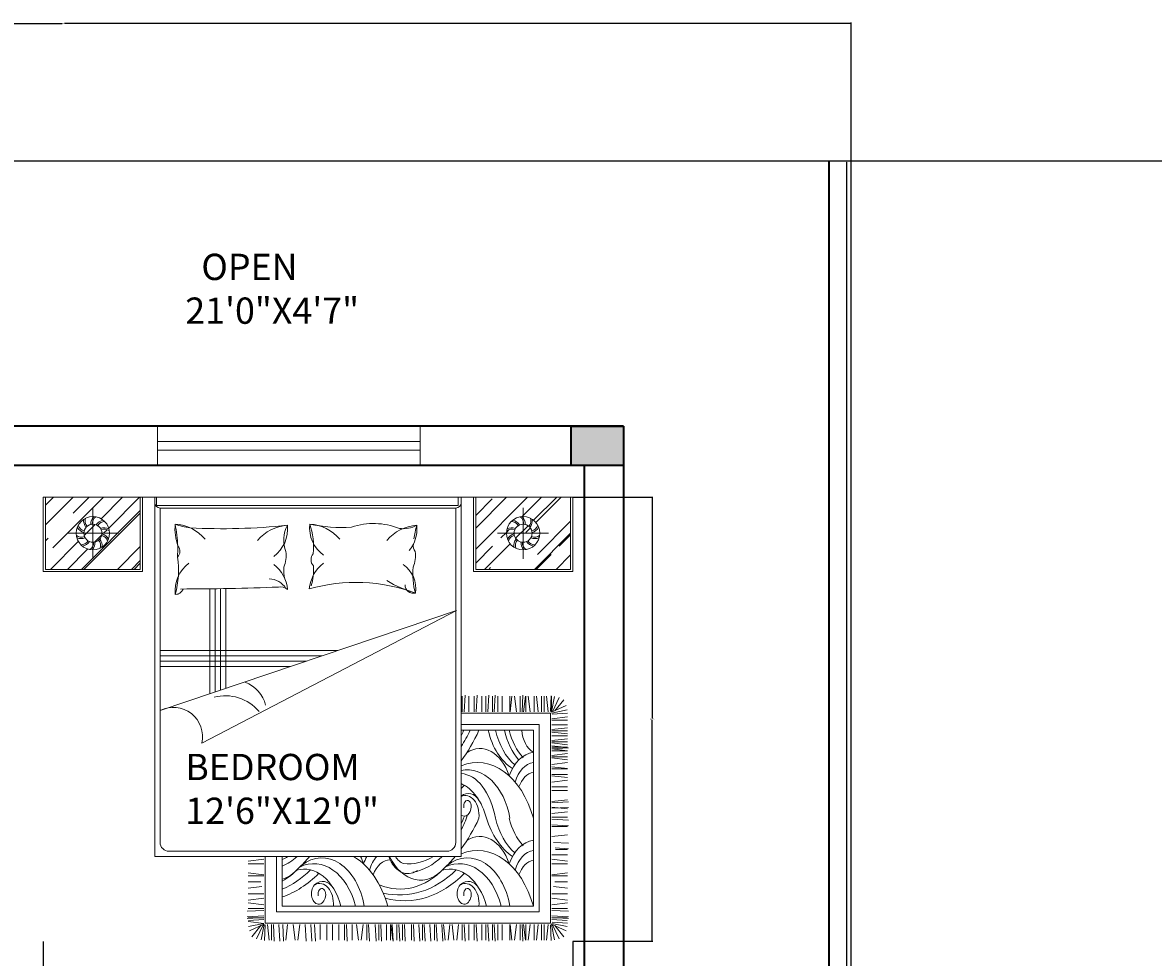
# Model space of a CAD drawing. Units: inches. Extents: x 1602 to 2642, y 1463 to 2270.
# Tile 4 of 5: x 1854 to 2113, y 1919 to 2132. Entities that reach past the tile are written whole.
import ezdxf

# ---------------------------------------------------------------- set-up
doc = ezdxf.new("R2010")
doc.units = ezdxf.units.IN
for name, color, linetype, lineweight in [('A-ANNO-DIMS', 2, 'Continuous', 18), ('A-AREA-IDEN', 7, 'Continuous', 18), ('A-COLS', 7, 'Continuous', 35), ('A-FURN', 8, 'Continuous', 13), ('A-GLAZ', 4, 'Continuous', 18), ('A-WALL', 7, 'Continuous', 35), ('C-PROP', 7, 'Continuous', 25)]:
    doc.layers.add(name, color=color, linetype=linetype, lineweight=lineweight)
doc.styles.get("Standard").update_dxf_attribs({"font": 'arial.ttf'})
doc.dimstyles.get("Standard").update_dxf_attribs({"dimtxt": 0.18, "dimasz": 0.18, "dimexe": 0.18, "dimexo": 0.0625, "dimgap": 0.09, "dimtad": 0, "dimtih": 1, "dimtoh": 1, "dimdec": 4, "dimzin": 0, "dimdsep": 46, "dimtxsty": 'Standard', "dimcen": 0.09, "dimadec": 0, "dimazin": 0, "dimtfac": 1, "dimtdec": 4, "dimtofl": 0, "dimtmove": 0, "dimatfit": 3, "dimfxl": 1, "dimtolj": 1, "dimtzin": 0, "dimarcsym": 0})

# ---------------------------------------------------------------- blocks, each defined once
blk = doc.blocks.new('A$C64B41DC1')
for p, q in [((0, 2.5079), (2.9903, 2.5079)), ((0, 2.0879), (0, 2.5079)), ((0.012, 2.4618), (0.0581, 2.5079)), ((0.012, 2.3515), (0.1684, 2.5079)), ((0.012, 2.0999), (0.012, 2.5079)), ((0.0543, 2.2213), (0.3409, 2.5079)), ((0.1689, 2.4179), (0.2589, 2.5079)), ((0.3265, 2.386), (0.4484, 2.5079)), ((0.3699, 2.3332), (0.5445, 2.5079)), ((0.548, 2.5079), (0.548, 2.0999)), ((0.56, 2.5079), (0.56, 2.0879)), ((0.6301, 2.5079), (0.6301, 0.4779)), ((0.6401, 2.461), (0.6401, 2.5079)), ((0.6401, 2.5079), (2.344, 2.5079)), ((2.344, 2.5079), (2.3601, 2.5079)), ((2.344, 2.5079), (2.344, 2.461)), ((2.3601, 2.5079), (2.3601, 2.4761)), ((2.3601, 0.4779), (2.3601, 2.5079)), ((2.4303, 2.5079), (2.4303, 2.0879)), ((2.4423, 2.5079), (2.4423, 2.0999)), ((2.4423, 2.3333), (2.6169, 2.5079)), ((2.4423, 2.2145), (2.7357, 2.5079)), ((2.4423, 2.404), (2.5354, 2.4971)), ((2.705, 2.398), (2.8149, 2.5079)), ((2.7691, 2.3772), (2.8998, 2.5079)), ((2.7819, 2.3646), (2.9252, 2.5079)), ((2.9783, 2.0999), (2.9783, 2.5079)), ((2.9903, 2.0879), (2.9903, 2.5079)), ((0.2157, 2.0999), (0.548, 2.4322)), ((0.2804, 2.1597), (0.2804, 2.4481)), ((2.344, 2.461), (0.6401, 2.461)), ((0.6601, 2.4461), (1.4951, 2.4461)), ((0.6601, 2.4461), (0.6601, 0.5579)), ((1.4951, 2.4461), (0.6697, 2.4461)), ((2.3301, 2.4461), (1.4951, 2.4461)), ((2.3301, 0.5579), (2.3301, 2.4461)), ((2.7099, 2.1597), (2.7099, 2.4481)), ((0.2299, 2.0999), (0.548, 2.418)), ((2.7914, 2.1846), (2.9783, 2.3715)), ((0.1362, 2.3039), (0.4246, 2.3039)), ((0.2311, 2.2906), (0.2937, 2.3532)), ((0.3405, 2.3039), (0.3605, 2.3238)), ((2.8541, 2.3039), (2.5657, 2.3039)), ((2.5849, 2.2779), (2.6158, 2.3088)), ((2.6158, 2.3088), (2.6313, 2.3243)), ((2.6674, 2.2756), (2.7382, 2.3464)), ((2.7249, 2.3076), (2.7512, 2.3339)), ((2.7746, 2.0999), (2.9783, 2.3036)), ((0.012, 2.261), (0.0275, 2.2765)), ((0.0404, 2.0999), (0.1982, 2.2578)), ((0.2905, 2.2539), (0.3304, 2.2938)), ((2.4918, 2.0999), (2.6366, 2.2447)), ((2.9144, 2.2312), (2.9783, 2.2951)), ((0.1365, 2.0999), (0.251, 2.2144)), ((0.4194, 2.0999), (0.548, 2.2285)), ((2.4423, 2.1353), (2.5382, 2.2312)), ((2.7831, 2.0999), (2.8678, 2.1846)), ((2.8962, 2.0999), (2.9783, 2.182)), ((0.4986, 2.0999), (0.548, 2.1493)), ((0.5127, 2.0999), (0.548, 2.1352)), ((2.5172, 2.0999), (2.5269, 2.1096)), ((0.56, 2.0879), (0, 2.0879)), ((0.548, 2.0999), (0.012, 2.0999)), ((2.4303, 2.0879), (2.9903, 2.0879)), ((2.4423, 2.0999), (2.9783, 2.0999)), ((0.9415, 1.9902), (0.9415, 1.3975)), ((0.9715, 1.9906), (0.9715, 1.4076)), ((1.0015, 1.991), (1.0015, 1.4177)), ((1.0315, 1.9916), (1.0315, 1.4279)), ((2.3349, 1.8678), (0.6613, 1.3029)), ((0.8956, 1.1191), (2.3349, 1.8678)), ((1.6636, 1.6412), (0.6601, 1.6412)), ((1.5748, 1.6112), (0.6601, 1.6112)), ((2.3665, 1.295), (2.3665, 1.3839)), ((2.377, 1.295), (2.3822, 1.3891)), ((2.4032, 1.295), (2.4032, 1.3839)), ((2.4346, 1.295), (2.4346, 1.3839)), ((2.4451, 1.295), (2.4503, 1.3891)), ((2.4774, 1.2957), (2.4774, 1.3837)), ((2.5, 1.295), (2.5, 1.3839)), ((2.5105, 1.295), (2.5157, 1.3891)), ((2.5367, 1.295), (2.5367, 1.3839)), ((2.5471, 1.295), (2.5524, 1.3891)), ((2.5681, 1.295), (2.5681, 1.3839)), ((2.5918, 1.295), (2.5918, 1.3839)), ((2.6346, 1.2957), (2.6346, 1.3837)), ((2.6362, 1.2957), (2.6467, 1.3839)), ((2.6729, 1.295), (2.6624, 1.3839)), ((2.6938, 1.295), (2.6938, 1.3839)), ((2.7043, 1.295), (2.7095, 1.3891)), ((2.7127, 1.2957), (2.7232, 1.3839)), ((2.7253, 1.295), (2.7253, 1.3839)), ((2.7494, 1.295), (2.7389, 1.3839)), ((2.7718, 1.295), (2.7718, 1.3839)), ((2.7959, 1.295), (2.7854, 1.3839)), ((2.8146, 1.2957), (2.8146, 1.3837)), ((2.8146, 1.2957), (2.8146, 1.3837)), ((2.8282, 1.295), (2.8282, 1.3839)), ((2.8282, 1.295), (2.8282, 1.3839)), ((2.8523, 1.295), (2.8418, 1.3839)), ((2.8523, 1.295), (2.8418, 1.3839)), ((2.8653, 1.2966), (2.8688, 1.3861)), ((2.8711, 1.2957), (2.8711, 1.3837)), ((2.8711, 1.2957), (2.8875, 1.3822)), ((2.8765, 1.2958), (2.9132, 1.3758)), ((2.8893, 1.3011), (2.9394, 1.3636)), ((2.3601, 1.2873), (2.8639, 1.2873)), ((2.8639, 1.2873), (2.8639, 0.1018)), ((2.8713, 1.2927), (2.954, 1.3315)), ((2.8717, 1.2884), (2.9588, 1.3058)), ((2.8744, 1.2817), (2.9603, 1.2869)), ((2.3601, 1.2233), (2.7999, 1.2233)), ((2.7999, 1.2233), (2.7999, 0.1658)), ((2.8716, 1.2565), (2.9605, 1.2669)), ((2.8716, 1.2212), (2.9605, 1.2212)), ((2.8723, 1.2489), (2.9603, 1.2489)), ((2.3601, 1.1913), (2.7679, 1.1912)), ((2.7679, 1.1912), (2.7679, 0.1978)), ((2.8716, 1.1947), (2.9605, 1.2052)), ((2.8716, 1.181), (2.9605, 1.1705)), ((2.8716, 1.1595), (2.9605, 1.1595)), ((2.8723, 1.1872), (2.9603, 1.1872)), ((2.8716, 1.133), (2.9605, 1.1435)), ((2.8716, 1.1193), (2.9605, 1.1088)), ((2.8716, 1.1035), (2.9605, 1.093)), ((2.8716, 1.0965), (2.9605, 1.0965)), ((2.8716, 1.086), (2.9657, 1.0913)), ((2.8723, 1.1255), (2.9603, 1.1255)), ((2.8723, 1.0858), (2.9605, 1.0753)), ((2.8716, 1.0756), (2.9605, 1.0756)), ((2.8716, 1.0491), (2.9605, 1.0596)), ((2.8716, 1.0354), (2.9605, 1.0249)), ((2.8723, 1.0416), (2.9603, 1.0416)), ((2.8723, 0.9987), (2.9605, 1.0092)), ((2.8723, 0.985), (2.9605, 0.9745)), ((2.8723, 0.9735), (2.9603, 0.9735)), ((2.8716, 0.9346), (2.9605, 0.9241)), ((2.8723, 0.9408), (2.9603, 0.9408)), ((2.8723, 0.8979), (2.9605, 0.9084)), ((2.8723, 0.8726), (2.9603, 0.8726)), ((2.8723, 0.8505), (2.9603, 0.8505)), ((2.8716, 0.7885), (2.9605, 0.799)), ((2.8716, 0.7818), (2.9657, 0.787)), ((2.8716, 0.7503), (2.9657, 0.7556)), ((2.8716, 0.7204), (2.9605, 0.7309)), ((2.8723, 0.7571), (2.9605, 0.7466)), ((2.8716, 0.6995), (2.9605, 0.6995)), ((2.8716, 0.689), (2.9657, 0.6838)), ((2.8716, 0.6576), (2.9657, 0.6523)), ((2.8716, 0.6471), (2.9605, 0.6471)), ((2.8716, 0.5903), (2.9605, 0.6007)), ((2.882, 0.5582), (2.9657, 0.5536)), ((2.8909, 0.5263), (2.9657, 0.5222)), ((2.8928, 0.5169), (2.9605, 0.5169)), ((0.6301, 0.4779), (2.3601, 0.4779)), ((0.7101, 0.5079), (2.2801, 0.5079)), ((1.2465, 0.4625), (1.1576, 0.452)), ((1.2542, 0.1018), (1.2542, 0.4779)), ((1.3182, 0.1658), (1.3182, 0.4779)), ((1.3502, 0.1978), (1.3502, 0.4779)), ((2.8716, 0.4877), (2.9603, 0.4877)), ((2.8716, 0.4625), (2.9605, 0.452)), ((1.2465, 0.3746), (1.1576, 0.3851)), ((1.2465, 0.4365), (1.1577, 0.4365)), ((2.8716, 0.4365), (2.9603, 0.4365)), ((2.8716, 0.3746), (2.9605, 0.3851)), ((1.2465, 0.3684), (1.1577, 0.3684)), ((1.2285, 0.3357), (1.1577, 0.3357)), ((2.8716, 0.3684), (2.9603, 0.3684)), ((2.8896, 0.3357), (2.9603, 0.3357)), ((1.2355, 0.3092), (1.1576, 0.3)), ((1.2457, 0.2676), (1.1577, 0.2676)), ((2.8723, 0.2676), (2.9603, 0.2676)), ((2.8826, 0.3092), (2.9605, 0.3)), ((1.2457, 0.2423), (1.1576, 0.2319)), ((1.2465, 0.2057), (1.1576, 0.2161)), ((2.7679, 0.1978), (1.3502, 0.1978)), ((2.8716, 0.2057), (2.9605, 0.2161)), ((2.8723, 0.2423), (2.9605, 0.2319)), ((1.2465, 0.1742), (1.1524, 0.169)), ((1.2465, 0.1428), (1.1524, 0.1376)), ((1.2465, 0.1334), (1.1524, 0.1281)), ((1.2465, 0.1847), (1.1576, 0.1847)), ((1.2465, 0.1323), (1.1576, 0.1323)), ((1.2465, 0.1323), (1.1576, 0.1323)), ((2.7999, 0.1658), (1.3182, 0.1658)), ((2.8716, 0.1847), (2.9605, 0.1847)), ((2.8716, 0.1742), (2.9657, 0.169)), ((2.8716, 0.1428), (2.9657, 0.1376)), ((2.8716, 0.1334), (2.9657, 0.1281)), ((2.8716, 0.1323), (2.9605, 0.1323)), ((1.2465, 0.1), (1.1576, 0.1105)), ((1.2465, 0.1229), (1.1588, 0.1168)), ((1.2464, 0.1007), (1.1592, 0.0833)), ((1.2468, 0.0964), (1.1641, 0.0576)), ((1.2288, 0.088), (1.1787, 0.0255)), ((1.2415, 0.0933), (1.2049, 0.0133)), ((1.247, 0.0934), (1.2306, 0.0069)), ((1.2527, 0.0925), (1.2493, 0.003)), ((2.8639, 0.1018), (1.2542, 0.1018)), ((1.2658, 0.0941), (1.2762, 0.0052)), ((1.2899, 0.0941), (1.2899, 0.0052)), ((1.2999, 0.0941), (1.3051, 0)), ((1.3313, 0.0941), (1.3365, 0)), ((1.3523, 0.0941), (1.3575, 0)), ((1.3804, 0.0941), (1.3699, 0.0052)), ((1.4119, 0.0934), (1.4223, 0.0052)), ((1.4485, 0.0941), (1.438, 0.0052)), ((1.48, 0.0941), (1.4852, 0)), ((1.5114, 0.0941), (1.5166, 0)), ((1.5323, 0.0941), (1.5376, 0)), ((1.5638, 0.0941), (1.5638, 0.0105)), ((1.6021, 0.0941), (1.6021, 0.0052)), ((1.6336, 0.0941), (1.6336, 0.0052)), ((1.6702, 0.0941), (1.6702, 0.0052)), ((1.7017, 0.0941), (1.7017, 0.0052)), ((1.7122, 0.0941), (1.7174, 0)), ((1.7445, 0.0934), (1.7445, 0.0054)), ((1.7698, 0.0934), (1.7803, 0.0052)), ((1.8065, 0.0941), (1.796, 0.0052)), ((1.8274, 0.0941), (1.8274, 0.0052)), ((1.8379, 0.0941), (1.8431, 0)), ((1.8746, 0.0941), (1.8798, 0)), ((1.8955, 0.0941), (1.8955, 0.0052)), ((1.906, 0.0941), (1.9113, 0)), ((1.9384, 0.0934), (1.9384, 0.0054)), ((1.9609, 0.0941), (1.9609, 0.0052)), ((1.9636, 0.0934), (1.9741, 0.0052)), ((1.9714, 0.0941), (1.9766, 0)), ((1.9976, 0.0941), (1.9976, 0.0052)), ((2.0081, 0.0941), (2.0133, 0)), ((2.029, 0.0941), (2.029, 0.0052)), ((2.0395, 0.0941), (2.0447, 0)), ((2.0797, 0.0941), (2.0797, 0.0052)), ((2.0902, 0.0941), (2.0954, 0)), ((2.1216, 0.0941), (2.1269, 0)), ((2.1412, 0.0941), (2.1412, 0.0052)), ((2.1517, 0.0941), (2.1569, 0)), ((2.1831, 0.0941), (2.1884, 0)), ((2.2093, 0.0941), (2.2093, 0.0052)), ((2.2198, 0.0941), (2.225, 0)), ((2.2512, 0.0941), (2.2565, 0)), ((2.2603, 0.0934), (2.2707, 0.0052)), ((2.2969, 0.0941), (2.2864, 0.0052)), ((2.3089, 0.0934), (2.3193, 0.0052)), ((2.3455, 0.0941), (2.3351, 0.0052)), ((2.3665, 0.0941), (2.3665, 0.0052)), ((2.377, 0.0941), (2.3822, 0)), ((2.4032, 0.0941), (2.4032, 0.0052)), ((2.4346, 0.0941), (2.4346, 0.0052)), ((2.4451, 0.0941), (2.4503, 0)), ((2.4774, 0.0934), (2.4774, 0.0054)), ((2.5, 0.0941), (2.5, 0.0052)), ((2.5105, 0.0941), (2.5157, 0)), ((2.5367, 0.0941), (2.5367, 0.0052)), ((2.5471, 0.0941), (2.5524, 0)), ((2.5681, 0.0941), (2.5681, 0.0052)), ((2.5918, 0.0941), (2.5918, 0.0052)), ((2.6346, 0.0934), (2.6346, 0.0054)), ((2.6362, 0.0934), (2.6467, 0.0052)), ((2.6729, 0.0941), (2.6624, 0.0052)), ((2.6938, 0.0941), (2.6938, 0.0052)), ((2.7043, 0.0941), (2.7095, 0)), ((2.7127, 0.0934), (2.7232, 0.0052)), ((2.7253, 0.0941), (2.7253, 0.0052)), ((2.7494, 0.0941), (2.7389, 0.0052)), ((2.7718, 0.0941), (2.7718, 0.0052)), ((2.7959, 0.0941), (2.7854, 0.0052)), ((2.8146, 0.0934), (2.8146, 0.0054)), ((2.8282, 0.0941), (2.8282, 0.0052)), ((2.8523, 0.0941), (2.8418, 0.0052)), ((2.8653, 0.0925), (2.8688, 0.003)), ((2.8711, 0.0934), (2.8875, 0.0069)), ((2.8713, 0.0964), (2.954, 0.0576)), ((2.8716, 0.1229), (2.9593, 0.1168)), ((2.8717, 0.1007), (2.9588, 0.0833)), ((2.8744, 0.1074), (2.9603, 0.1022)), ((2.8765, 0.0933), (2.9132, 0.0133)), ((2.8893, 0.088), (2.9394, 0.0255))]:
    blk.add_line(p, q)
at = {"ltscale": 10}
for p, q in [((1.4859, 1.5812), (0.6601, 1.5812)), ((1.397, 1.5512), (0.6601, 1.5512))]:
    blk.add_line(p, q, dxfattribs=at)
for centre, radius in [((0.2804, 2.3039), 0.0942), ((2.7099, 2.3039), 0.0942), ((0.2804, 2.3039), 0.051), ((2.7099, 2.3039), 0.051)]:
    blk.add_circle(centre, radius)
for centre, radius, start, end in [((0.6601, 2.4761), 0.03, 180, 270), ((2.3301, 2.4761), 0.03, 270, 0), ((0.2887, 2.3745), 0.0605, 172.17003, 218.48975), ((0.2828, 2.3731), 0.0462, 160.30017, 220.53802), ((0.3286, 2.3561), 0.0605, 136.17003, 182.48975), ((0.3231, 2.3585), 0.0462, 124.30017, 184.53802), ((0.3501, 2.3178), 0.0605, 100.17003, 146.48975), ((0.347, 2.323), 0.0462, 88.30017, 148.53802), ((2.6433, 2.323), 0.0462, 31.46198, 91.69983), ((2.6402, 2.3178), 0.0605, 33.51025, 79.82997), ((2.6672, 2.3585), 0.0462, 355.46198, 55.69983), ((2.6617, 2.3561), 0.0605, 357.51025, 43.82997), ((2.7075, 2.3731), 0.0462, 319.46198, 19.69983), ((2.7016, 2.3745), 0.0605, 321.51025, 7.82997), ((0.2457, 2.3659), 0.0605, 208.17003, 254.48975), ((0.2417, 2.3614), 0.0462, 196.30017, 256.53802), ((0.3449, 2.2742), 0.0605, 64.17003, 110.48975), ((0.3455, 2.2802), 0.0462, 52.30017, 112.53802), ((0.3151, 2.2419), 0.0605, 28.17003, 74.48975), ((1.0526, 2.3302), 0.3085, 175.30484, 198.69419), ((-0.8702, 2.0941), 1.6364, 4.80985, 9.18918), ((0.8579, 2.6278), 0.2948, 247.51785, 264.26696), ((0.728, 2.111), 0.245, 40.4189, 85.9871), ((1.0164, 5.7096), 3.3803, 266.81337, 276.16021), ((1.3963, 2.1044), 0.245, 94.0129, 139.5811), ((1.1858, 2.3288), 0.1943, 306.5711, 5.88998), ((1.5348, 2.2652), 0.1767, 151.77364, 201.69827), ((1.6986, 2.3355), 0.1943, 174.11002, 233.4289), ((1.1481, 2.2311), 0.3783, 353.49469, 19.18669), ((1.6871, 3.192), 0.8561, 257.74383, 273.62843), ((1.4882, 2.111), 0.245, 40.4189, 85.9871), ((1.8674, 1.9709), 0.3878, 68.20259, 108.9817), ((2.1269, 2.1044), 0.245, 94.0129, 139.5811), ((2.0342, 2.4856), 0.1563, 261.59582, 298.90918), ((1.9165, 2.3288), 0.1943, 333.73715, 5.88998), ((2.6058, 2.2028), 0.517, 163.60457, 172.3273), ((2.6448, 2.2802), 0.0462, 67.46198, 127.69983), ((2.6454, 2.2742), 0.0605, 69.51025, 115.82997), ((2.6752, 2.2419), 0.0605, 105.51025, 151.82997), ((2.7486, 2.3614), 0.0462, 283.46198, 343.69983), ((2.7446, 2.3659), 0.0605, 285.51025, 331.82997), ((0.2153, 2.3276), 0.0462, 232.30017, 292.53802), ((0.2158, 2.3336), 0.0605, 244.17003, 290.48975), ((0.2138, 2.2848), 0.0462, 268.30017, 328.53802), ((0.2107, 2.29), 0.0605, 280.17003, 326.48975), ((0.2377, 2.2493), 0.0462, 304.30017, 4.53802), ((0.2322, 2.2517), 0.0605, 316.17003, 2.48975), ((0.2779, 2.2347), 0.0462, 340.30017, 40.53802), ((0.272, 2.2333), 0.0605, 352.17003, 38.48975), ((0.3191, 2.2464), 0.0462, 16.30017, 76.53802), ((1.9165, 2.3288), 0.1943, 320.94042, 333.73715), ((2.1347, 2.2313), 0.0459, 165.35061, 223.26844), ((2.6712, 2.2464), 0.0462, 103.46198, 163.69983), ((2.7182, 2.2333), 0.0605, 141.51025, 187.82997), ((2.7123, 2.2347), 0.0462, 139.46198, 199.69983), ((2.7581, 2.2517), 0.0605, 177.51025, 223.82997), ((2.7526, 2.2493), 0.0462, 175.46198, 235.69983), ((2.7796, 2.29), 0.0605, 213.51025, 259.82997), ((2.7765, 2.2848), 0.0462, 211.46198, 271.69983), ((2.7744, 2.3336), 0.0605, 249.51025, 295.82997), ((2.775, 2.3276), 0.0462, 247.46198, 307.69983), ((0.7274, 2.2013), 0.0446, 314.4736, 42.17134), ((-1.6008, 2.277), 2.3618, 357.39054, 358.88764), ((1.204, 2.1778), 0.1681, 337.01697, 7.53676), ((1.5671, 2.1546), 0.0547, 142.08329, 220.902), ((1.9346, 2.1778), 0.1681, 337.01697, 7.53676), ((0.9385, 1.978), 0.1943, 126.5711, 185.88998), ((0.2688, 2.0945), 0.4956, 344.0243, 8.70709), ((1.1858, 1.9714), 0.1943, 4.31813, 53.4289), ((1.5415, 2.0969), 0.1834, 175.22328, 196.23004), ((1.7059, 1.9714), 0.204, 127.11975, 175.09005), ((1.1965, 2.0983), 0.3299, 343.79543, 3.55541), ((1.9394, 1.991), 0.1651, 351.26213, 55.75721), ((2.4617, 2.0719), 0.3745, 173.82958, 196.4356), ((1.2687, 1.9248), 0.1223, 33.62799, 86.47438), ((0.7417, 2.0149), 0.057, 273.47085, 328.54118), ((0.7246, 18.8439), 16.8552, 270.17399, 272.05214), ((1.3401, 1.9404), 0.0603, 49.09906, 101.37023), ((1.7676, 1.0629), 0.9631, 69.65065, 105.96307), ((2.2748, 2.5795), 0.6373, 238.34989, 254.31375), ((2.0911, 2.0123), 0.0478, 179.77267, 283.80184), ((0.728, 2.2025), 0.245, 274.0129, 278.34166), ((1.0747, 1.2871), 0.1871, 14.1863, 69.12121), ((1.0274, 1.1334), 0.2527, 40.62904, 104.37123), ((0.7347, 1.1553), 0.1649, 347.31088, 116.44537), ((0.7101, 0.5579), 0.05, 180, 270), ((2.2801, 0.5579), 0.05, 270, 0)]:
    blk.add_arc(centre, radius, start, end)
for centre, major_axis, ratio, start_param, end_param in [((1.9938, 1.6262), (0, -0.7531), 0.68, 0.797284, 0.954936), ((2.0643, 1.466), (0, -0.5322), 0.68, 7.239912, 7.311536), ((1.9052, 1.7397), (0, -0.9842), 0.68, 0.74745, 0.979724), ((2.7455, 1.3081), (0, 0.3614), 0.68, 1.900046, 2.742661), ((2.7868, 1.3081), (0, 0.3614), 0.68, 1.900046, 2.614747), ((2.8372, 1.3081), (0, 0.3614), 0.68, 1.900046, 2.479658), ((2.8607, 1.3211), (0, 0.3614), 0.68, 1.938265, 2.479658), ((2.8057, 1.2079), (0, -0.1524), 0.68, 4.821745, 5.895886), ((2.4665, 0.8216), (0, -0.2664), 0.68, 2.006169, 3.565187), ((2.4513, 0.5069), (0, 0.502), 0.68, 5.095327, 6.553458), ((2.7862, 0.8069), (0, -0.2615), 0.68, 3.244645, 4.205018), ((2.396, 0.6032), (0, 0.3641), 0.68, -1.3172, 0.145284), ((2.7784, 0.8289), (0, -0.1802), 0.68, 3.227058, 4.318474), ((2.3507, 0.5642), (0.0073, 0.3819), 0.56205, -1.21172, -0.009991), ((2.7821, 0.7971), (0, -0.1589), 0.68, 3.272942, 4.229533), ((2.2964, 0.5771), (0, -0.3263), 0.68, 1.938944, 2.850232), ((2.0403, 1.6015), (0, -0.8763), 0.68, 6.849801, 6.887077), ((2.4005, 0.7132), (0, -0.1214), 0.68, 2.284368, 3.652258), ((2.3834, 0.7081), (0, 0.1147), 0.68, 4.593909, 6.585576), ((2.3961, 0.7628), (0, -0.0317), 0.68, 1.462497, 5.046281), ((2.3774, 0.7653), (0, -0.0593), 0.68, 5.841311, 7.755362), ((1.9938, 1.1295), (-0.0678, 0.7439), 0.610498, 3.917146, 4.063997), ((2.0643, 0.9693), (0, -0.5322), 0.68, 7.239912, 7.336618), ((1.9052, 1.243), (0, -0.9842), 0.68, 0.74745, 0.979724), ((2.7455, 0.8114), (-0.0599, 0.3735), 0.695517, 1.775813, 2.548612), ((2.7868, 0.8114), (0, 0.3614), 0.68, 1.900046, 2.614747), ((2.8607, 0.8243), (0, 0.3614), 0.68, 1.938265, 2.479658), ((2.4665, 0.3249), (0, -0.2664), 0.68, 2.006169, 3.565187), ((2.4513, 0.0102), (0, 0.502), 0.68, 5.095327, 6.553458), ((2.7862, 0.3102), (0, -0.2615), 0.68, 3.244645, 4.205018), ((2.7784, 0.3322), (0, -0.1802), 0.68, 3.227058, 4.318474), ((1.242, 0.9693), (0, -0.5322), 0.68, 6.586764, 6.677612), ((1.1714, 1.1295), (-0.1157, 0.7241), 0.59432, 3.291697, 3.50733), ((1.0828, 1.243), (0, -0.9842), 0.68, 0.565948, 0.680366), ((1.5283, 0.0674), (0, -0.3703), 0.68, 1.930561, 3.464283), ((1.5736, 0.1065), (0, 0.3641), 0.68, -1.3172, 0.476403), ((1.6289, 0.0102), (0, 0.502), 0.68, 6.655152, 6.661293), ((1.6289, 0.0102), (0, 0.502), 0.68, 5.095327, 5.911219), ((1.6442, 0.3249), (0, -0.2664), 0.68, 2.006169, 2.182797), ((1.9638, 0.3102), (0, -0.2615), 0.68, 4.015924, 4.205018), ((1.956, 0.3322), (0, -0.1802), 0.68, 3.770744, 4.318474), ((1.9597, 0.3004), (0, -0.1589), 0.68, 3.14258, 4.229533), ((2.0606, 0.5616), (0, -0.1803), 0.68, 5.194792, 5.929328), ((2.0606, 0.5616), (0, -0.1803), 0.68, 5.194792, 6.723255), ((2.1315, 0.6603), (0, -0.3155), 0.68, 5.328638, 6.949396), ((2.0549, 0.5656), (0, -0.1303), 0.68, 5.450951, 6.054641), ((2.0643, 0.9693), (0, -0.5322), 0.68, 6.20013, 6.677612), ((1.9938, 1.1295), (-0.0678, 0.7439), 0.610498, 3.199135, 3.592282), ((1.9052, 1.243), (0, -0.9842), 0.68, 0.565948, 0.680366), ((2.3507, 0.0674), (0, -0.3703), 0.68, 1.930561, 3.464283), ((2.396, 0.1065), (0, 0.3641), 0.68, -1.3172, 0.476403), ((2.4513, 0.0102), (0, 0.502), 0.68, 6.655152, 6.661293), ((2.7821, 0.3004), (0, -0.1589), 0.68, 3.272942, 4.229533), ((1.1933, 0.9181), (0, -0.624), 0.68, 0.378672, 0.625379), ((1.3091, 0.6603), (0, -0.3155), 0.68, 6.475719, 6.949396), ((1.1911, 1.1066), (0, 0.8458), 0.68, 3.421828, 3.728616), ((1.2179, 1.1047), (0, -0.8763), 0.68, 6.507006, 6.887077), ((1.474, 0.0804), (0, -0.3263), 0.68, 1.938944, 3.339184), ((2.0157, 0.9181), (0, -0.624), 0.68, -0.280078, 0.625379), ((2.0135, 1.1066), (0, 0.8458), 0.68, 2.978727, 3.728616), ((2.0403, 1.1047), (0, -0.8763), 0.68, 6.099302, 6.887077), ((2.2964, 0.0804), (0, -0.3263), 0.68, 1.938944, 3.339184), ((1.5781, 0.2165), (0, -0.1214), 0.68, 2.284368, 3.726131), ((1.561, 0.2114), (0, 0.1147), 0.68, 4.593909, 6.647252), ((2.4005, 0.2165), (0, -0.1214), 0.68, 2.284368, 3.726131), ((2.3834, 0.2114), (0, 0.1147), 0.68, 4.593909, 6.647252), ((1.555, 0.2685), (0, -0.0593), 0.68, 3.732151, 7.755362), ((1.5737, 0.2661), (0, -0.0317), 0.68, 1.462497, 5.046281), ((2.3774, 0.2685), (0, -0.0593), 0.68, 3.732151, 7.755362), ((2.3961, 0.2661), (0, -0.0317), 0.68, 1.462497, 5.046281)]:
    blk.add_ellipse(centre, major_axis=major_axis, ratio=ratio, start_param=start_param, end_param=end_param)
blk = doc.blocks.new('WIN-60IN')
for p, q in [((0, 0), (0, 9)), ((60, 0), (60, 9)), ((60, 5.5), (0, 5.5)), ((60, 3.5), (0, 3.5))]:
    blk.add_line(p, q)
blk = doc.blocks.new('COL-12X9')
h = blk.add_hatch(color=256)
h.dxf.hatch_style = 1
h.paths.add_polyline_path([(12, 0), (12, 9), (0, 9), (0, 0)])
blk.add_lwpolyline([(12, 9), (12, 0), (0, 0), (0, 9)], close=True)
blk = doc.blocks.new('*D15')
at = {"layer": 'A-ANNO-DIMS', "color": 0, "lineweight": -2, "transparency": 16777216}
for p, q in [((1859.14, 1922.53), (1859.14, 1904.26)), ((1980.1, 1922.53), (1980.1, 1904.26)), ((1859.32, 1904.44), (1918.45, 1904.44)), ((1979.92, 1904.44), (1920.79, 1904.44))]:
    blk.add_line(p, q, dxfattribs=at)
at = {"layer": 'A-ANNO-DIMS', "color": 0, "transparency": 16777216}
for points in [[(1859.32, 1904.47), (1859.32, 1904.41), (1859.14, 1904.44)], [(1979.92, 1904.47), (1979.92, 1904.41), (1980.1, 1904.44)]]:
    blk.add_solid(points, dxfattribs=at)
at = {"layer": 'Defpoints', "color": 0, "transparency": 16777216}
for p in [(1859.14, 1922.59), (1980.1, 1922.59), (1980.1, 1904.44)]:
    blk.add_point(p, dxfattribs=at)
at = {"layer": 'A-ANNO-DIMS', "color": 0, "transparency": 16777216, "insert": (1919.62, 1904.44), "char_height": 0.18, "attachment_point": 5}
blk.add_mtext('\\A1;BED SET 121 TYP.', dxfattribs=at)
blk = doc.blocks.new('*D16')
at = {"layer": 'A-ANNO-DIMS', "color": 0, "lineweight": -2, "transparency": 16777216}
for p, q in [((1980.17, 2024.04), (1998.43, 2024.04)), ((1998.25, 2023.86), (1998.25, 1973.5)), ((1998.25, 1922.77), (1998.25, 1973.13)), ((1980.17, 1922.59), (1998.43, 1922.59))]:
    blk.add_line(p, q, dxfattribs=at)
at = {"layer": 'A-ANNO-DIMS', "color": 0, "transparency": 16777216}
for points in [[(1998.22, 2023.86), (1998.28, 2023.86), (1998.25, 2024.04)], [(1998.22, 1922.77), (1998.28, 1922.77), (1998.25, 1922.59)]]:
    blk.add_solid(points, dxfattribs=at)
at = {"layer": 'Defpoints', "color": 0, "transparency": 16777216}
for p in [(1980.1, 2024.04), (1998.25, 2024.04), (1980.1, 1922.59)]:
    blk.add_point(p, dxfattribs=at)
at = {"layer": 'A-ANNO-DIMS', "color": 0, "transparency": 16777216, "insert": (1998.25, 1973.31), "char_height": 0.18, "attachment_point": 5}
blk.add_mtext('\\A1;101 TYP.', dxfattribs=at)
blk = doc.blocks.new('*D39')
at = {"layer": 'A-ANNO-DIMS', "color": 0, "lineweight": -2, "transparency": 16777216}
for p, q in [((1683.73, 2100.81), (1683.73, 2132.43)), ((1683.91, 2132.25), (1863.44, 2132.25)), ((2043.55, 2132.25), (1864.02, 2132.25)), ((2043.73, 2100.81), (2043.73, 2132.43))]:
    blk.add_line(p, q, dxfattribs=at)
at = {"layer": 'A-ANNO-DIMS', "color": 0, "transparency": 16777216}
for points in [[(1683.91, 2132.28), (1683.91, 2132.22), (1683.73, 2132.25)], [(2043.55, 2132.28), (2043.55, 2132.22), (2043.73, 2132.25)]]:
    blk.add_solid(points, dxfattribs=at)
at = {"layer": 'Defpoints', "color": 0, "transparency": 16777216}
for p in [(2043.73, 2132.25), (1683.73, 2100.75), (2043.73, 2100.75)]:
    blk.add_point(p, dxfattribs=at)
at = {"layer": 'A-ANNO-DIMS', "color": 0, "transparency": 16777216, "insert": (1863.73, 2132.25), "char_height": 0.18, "attachment_point": 5}
blk.add_mtext('\\A1;360', dxfattribs=at)
blk = doc.blocks.new('*D42')
at = {"layer": 'A-ANNO-DIMS', "color": 0, "lineweight": -2, "transparency": 16777216}
for p, q in [((2130.59, 2100.75), (2042.46, 2100.75)), ((2042.64, 2100.57), (2042.64, 1800.93)), ((2042.64, 1500.93), (2042.64, 1800.57)), ((2130.59, 1500.75), (2042.46, 1500.75))]:
    blk.add_line(p, q, dxfattribs=at)
at = {"layer": 'A-ANNO-DIMS', "color": 0, "transparency": 16777216}
for points in [[(2042.61, 2100.57), (2042.67, 2100.57), (2042.64, 2100.75)], [(2042.61, 1500.93), (2042.67, 1500.93), (2042.64, 1500.75)]]:
    blk.add_solid(points, dxfattribs=at)
at = {"layer": 'Defpoints', "color": 0, "transparency": 16777216}
for p in [(2042.64, 2100.75), (2130.66, 2100.75), (2130.66, 1500.75)]:
    blk.add_point(p, dxfattribs=at)
at = {"layer": 'A-ANNO-DIMS', "color": 0, "transparency": 16777216, "insert": (2042.64, 1800.75), "char_height": 0.18, "attachment_point": 5}
blk.add_mtext('\\A1;600', dxfattribs=at)

msp = doc.modelspace()

# ---------------------------------------------------------------- linework, layer by layer
at = {"layer": 'A-WALL'}
for p, q in [((2038.73, 1734.25), (2038.73, 2100.75)), ((1991.73, 2040.25), (1781.73, 2040.25)), ((1991.73, 2040.25), (1991.73, 1725.25)), ((1982.73, 2031.25), (1847.73, 2031.25)), ((1982.73, 2031.25), (1982.73, 1887.25))]:
    msp.add_line(p, q, dxfattribs=at)
at = {"layer": 'C-PROP'}
for p, q in [((2043.73, 2100.75), (1683.73, 2100.75)), ((2043.73, 1500.75), (2043.73, 2100.75))]:
    msp.add_line(p, q, dxfattribs=at)

# ---------------------------------------------------------------- block references
at = {"layer": 'A-COLS'}
msp.add_blockref('COL-12X9', (1979.73, 2031.25), dxfattribs=at)
at = {"layer": 'A-FURN', "xscale": 40.4528793712771, "yscale": 40.4528793712771, "zscale": 40.4528793712771}
msp.add_blockref('A$C64B41DC1', (1859.14, 1922.59), dxfattribs=at)
at = {"layer": 'A-GLAZ'}
msp.add_blockref('WIN-60IN', (1885.23, 2031.25), dxfattribs=at)

# ---------------------------------------------------------------- texts
at = {"layer": 'A-AREA-IDEN', "char_height": 6, "attachment_point": 1}
for s, insert in [('  OPEN\\P21\'0"X4\'7"', (1891.59, 2079.63)), ('BEDROOM\\P12\'6"X12\'0"', (1891.59, 1965.38))]:
    msp.add_mtext_dynamic_manual_height_columns(s, width=107.2848, gutter_width=12.5, heights=[0], dxfattribs=dict(at, insert=insert))

# ---------------------------------------------------------------- dimensions: what is measured, and where the dimension line sits
at = {"layer": 'A-ANNO-DIMS'}
dim = msp.add_linear_dim(base=(2043.73, 2132.25), p1=(1683.73, 2100.75), p2=(2043.73, 2100.75), dimstyle='Standard', override={"dimdec": 0, "dimlfac": 1, "dimrnd": 0, "dimzin": 0, "dimdsep": 46, "dimlunit": 2}, dxfattribs=at)
dim.commit()
dim.dimension.update_dxf_attribs({"geometry": '*D39', "text_midpoint": (1863.73, 2132.25)})
dim = msp.add_linear_dim(base=(2042.64, 2100.75), p1=(2130.66, 1500.75), p2=(2130.66, 2100.75), angle=90, dimstyle='Standard', override={"dimdec": 0, "dimlfac": 1, "dimrnd": 0, "dimzin": 0, "dimdsep": 46, "dimlunit": 2}, dxfattribs=at)
dim.commit()
dim.dimension.update_dxf_attribs({"geometry": '*D42', "text_midpoint": (2042.64, 1800.75)})
dim = msp.add_linear_dim(base=(1998.25, 2024.04), p1=(1980.1, 1922.59), p2=(1980.1, 2024.04), angle=90, text='<> TYP.', dimstyle='Standard', override={"dimdec": 0, "dimlfac": 1, "dimrnd": 0, "dimzin": 0, "dimdsep": 46, "dimlunit": 2}, dxfattribs=at)
dim.commit()
dim.dimension.update_dxf_attribs({"geometry": '*D16', "text_midpoint": (1998.25, 1973.31)})
dim = msp.add_linear_dim(base=(1980.1, 1904.44), p1=(1859.14, 1922.59), p2=(1980.1, 1922.59), text='BED SET <> TYP.', dimstyle='Standard', override={"dimdec": 0, "dimlfac": 1, "dimrnd": 0, "dimzin": 0, "dimdsep": 46, "dimlunit": 2}, dxfattribs=at)
dim.commit()
dim.dimension.update_dxf_attribs({"geometry": '*D15', "text_midpoint": (1919.62, 1904.44)})

doc.saveas('drawing.dxf')
